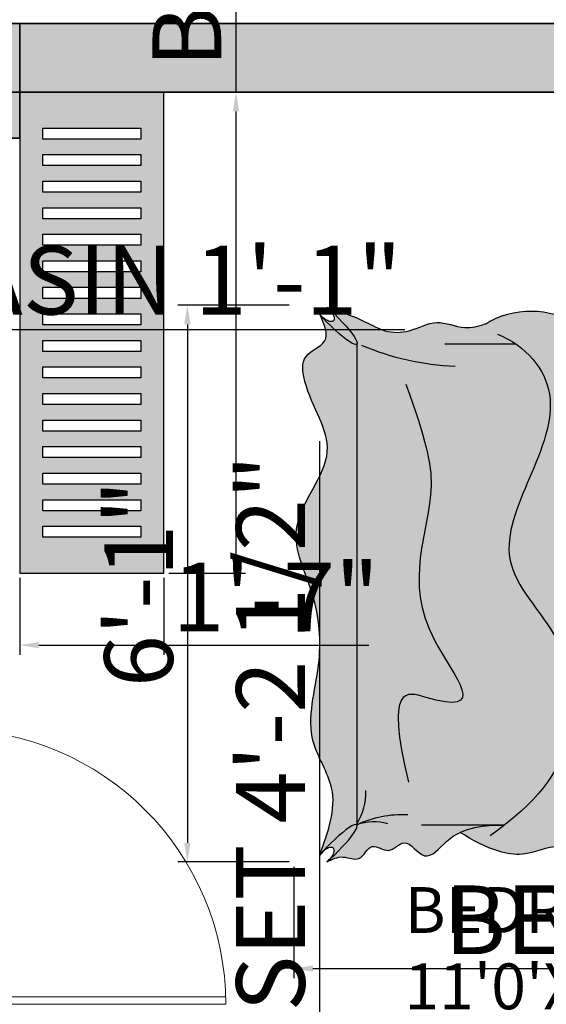
# Model space of a CAD drawing. Units: inches. Extents: x 3148 to 3962, y 1142 to 1671.
# Tile 4 of 9: x 3344 to 3413, y 1426 to 1555. Entities that reach past the tile are written whole.
import ezdxf

# ---------------------------------------------------------------- set-up
doc = ezdxf.new("R2010")
doc.units = ezdxf.units.IN
for name, color, linetype, lineweight in [('A-ANNO-DIMS', 2, 'Continuous', 18), ('A-AREA-IDEN', 7, 'Continuous', 18), ('A-COLS', 1, 'Continuous', 35), ('A-DOOR', 3, 'Continuous', 18), ('A-FURN', 8, 'Continuous', 18), ('A-WALL', 7, 'Continuous', 35), ('estofado', 7, 'Continuous', 25)]:
    doc.layers.add(name, color=color, linetype=linetype, lineweight=lineweight)
doc.layers.add('A-WALL-PATT', color=252, linetype='Continuous', lineweight=13, true_color=0x939598)
doc.layers.add('MESA', color=7, linetype='Continuous')
doc.styles.get("Standard").update_dxf_attribs({"font": 'arial.ttf'})
doc.dimstyles.new('ISO-25', dxfattribs={"dimtxt": 9, "dimasz": 2.5, "dimexe": 1.25, "dimexo": 0.625, "dimtad": 1, "dimdec": 1, "dimlunit": 3, "dimtxsty": 'Standard', "dimcen": 2.5, "dimadec": 0, "dimazin": 0, "dimtfac": 1, "dimtdec": 1, "dimtmove": 0, "dimatfit": 3, "dimfxl": 1, "dimarcsym": 0})

# ---------------------------------------------------------------- blocks, each defined once
blk = doc.blocks.new('Banco Lintz')
at = {"layer": 'MESA', "ltscale": 0.05}
h = blk.add_hatch(color=256, dxfattribs=at)
h.dxf.hatch_style = 1
h.set_gradient(color1=(138, 84, 66), color2=(0, 0, 0), one_color=1, name='INVCYLINDER')
h.paths.add_polyline_path([(0.4800000000000182, 0), (0, -5.68e-14), (0, -1.600000000000079), (0.4800000000000182, -1.600000000000079)])
h.paths.add_polyline_path([(0.403418045995295, -0.5090567265236814), (0.0765819540050643, -0.5090567265236245), (0.076581954005178, -0.4724032111287216), (0.4034180459950676, -0.4724032111288921)], flags=16)
h.paths.add_polyline_path([(0.4034180459950676, -0.5607660771784709), (0.4034180459950676, -0.597419592573317), (0.076581954005178, -0.597419592573317), (0.076581954005178, -0.560766077178414)], flags=16)
h.paths.add_polyline_path([(0.4034180459951813, -0.420693860473989), (0.0765819540050643, -0.420693860473989), (0.076581954005178, -0.3840403450791427), (0.4034180459950676, -0.3840403450791427)], flags=16)
h.paths.add_polyline_path([(0.4034180459950676, -0.6491289432280496), (0.4034180459950676, -0.6857824586229527), (0.076581954005178, -0.6857824586229527), (0.0765819540050643, -0.6491289432281065)], flags=16)
h.paths.add_polyline_path([(0.4034180459949539, -0.3323309944244102), (0.076581954005178, -0.3323309944244102), (0.0765819540050643, -0.2956774790295071), (0.4034180459950676, -0.2956774790295071)], flags=16)
h.paths.add_polyline_path([(0.4034180459950676, -0.737491809277742), (0.4034180459950676, -0.7741453246725883), (0.076581954005178, -0.7741453246725883), (0.0765819540050643, -0.737491809277742)], flags=16)
h.paths.add_polyline_path([(0.4034180459950676, -0.2439681283747745), (0.076581954005178, -0.2439681283747177), (0.076581954005178, -0.2073146129798147), (0.4034180459950676, -0.2073146129799284)], flags=16)
h.paths.add_polyline_path([(0.4034180459950676, -0.8258546753271502), (0.4034180459950676, -0.8625081907222238), (0.076581954005178, -0.86250819072211), (0.0765819540050643, -0.8258546753274913)], flags=16)
h.paths.add_polyline_path([(0.4034180459951813, -0.1556052623250821), (0.0765819540050643, -0.1556052623250252), (0.0765819540049506, -0.1189517469303496), (0.4034180459951813, -0.1189517469302928)], flags=16)
h.paths.add_polyline_path([(0.4034180459950676, -0.9142175413771269), (0.4034180459949539, -0.9508710567719163), (0.076581954005178, -0.9508710567718026), (0.076581954005178, -0.9142175413769564)], flags=16)
h.paths.add_polyline_path([(0.4034180459950676, -1.002580407426705), (0.4034180459951813, -1.039233922821438), (0.0765819540050643, -1.039233922821438), (0.076581954005178, -1.002580407426592)], flags=16)
h.paths.add_polyline_path([(0.4034180459950676, -1.090943273476284), (0.4034180459950676, -1.127596788871073), (0.076581954005178, -1.127596788871016), (0.0765819540049506, -1.090943273476284)], flags=16)
h.paths.add_polyline_path([(0.4034180459950676, -1.17930613952592), (0.4034180459950676, -1.215959654920709), (0.076581954005178, -1.215959654920709), (0.076581954005178, -1.179306139525806)], flags=16)
h.paths.add_polyline_path([(0.4034180459950676, -1.267669005575498), (0.4034180459950676, -1.304322520970401), (0.076581954005178, -1.304322520970345), (0.076581954005178, -1.267669005575498)], flags=16)
h.paths.add_polyline_path([(0.4034180459950676, -1.356031871625077), (0.4034180459950676, -1.392685387020094), (0.076581954005178, -1.39268538701998), (0.076581954005178, -1.356031871625134)], flags=16)
h.paths.add_polyline_path([(0.4034180459950676, -1.444394737673064), (0.4034180459950676, -1.481048253069729), (0.076581954005178, -1.481048253069616), (0.076581954005178, -1.444394737674826)], flags=16)
for points in [[(0, -1.600000000000022), (0.4800000000000182, -1.600000000000022), (0.4800000000000182, 0), (0, 0)], [(0.0765819540050643, -0.1189517469302928), (0.4034180459950676, -0.1189517469302928), (0.4034180459950676, -0.1556052623251389), (0.0765819540050643, -0.1556052623251389)], [(0.0765819540050643, -0.2073146129799284), (0.4034180459950676, -0.2073146129799284), (0.4034180459950676, -0.2439681283747745), (0.0765819540050643, -0.2439681283747745)], [(0.0765819540050643, -0.295677479029564), (0.4034180459950676, -0.295677479029564), (0.4034180459950676, -0.3323309944244102), (0.0765819540050643, -0.3323309944244102)], [(0.0765819540050643, -0.3840403450791996), (0.4034180459950676, -0.3840403450791996), (0.4034180459950676, -0.4206938604740458), (0.0765819540050643, -0.4206938604740458)], [(0.0765819540050643, -0.4724032111288352), (0.4034180459950676, -0.4724032111288352), (0.4034180459950676, -0.5090567265236814), (0.0765819540050643, -0.5090567265236814)], [(0.0765819540050643, -0.5607660771784709), (0.4034180459950676, -0.5607660771784709), (0.4034180459950676, -0.597419592573317), (0.0765819540050643, -0.597419592573317)], [(0.0765819540050643, -0.6491289432281065), (0.4034180459950676, -0.6491289432281065), (0.4034180459950676, -0.6857824586229527), (0.0765819540050643, -0.6857824586229527)], [(0.0765819540050643, -0.737491809277742), (0.4034180459950676, -0.737491809277742), (0.4034180459950676, -0.7741453246725883), (0.0765819540050643, -0.7741453246725883)], [(0.0765819540050643, -0.8258546753273776), (0.4034180459950676, -0.8258546753273776), (0.4034180459950676, -0.8625081907222238), (0.0765819540050643, -0.8625081907222238)], [(0.0765819540050643, -0.9142175413770132), (0.4034180459950676, -0.9142175413770132), (0.4034180459950676, -0.9508710567718593), (0.0765819540050643, -0.9508710567718593)], [(0.0765819540050643, -1.002580407426648), (0.4034180459950676, -1.002580407426648), (0.4034180459950676, -1.039233922821495), (0.0765819540050643, -1.039233922821495)], [(0.0765819540050643, -1.090943273476284), (0.4034180459950676, -1.090943273476284), (0.4034180459950676, -1.12759678887113), (0.0765819540050643, -1.12759678887113)], [(0.0765819540050643, -1.17930613952592), (0.4034180459950676, -1.17930613952592), (0.4034180459950676, -1.215959654920766), (0.0765819540050643, -1.215959654920766)], [(0.0765819540050643, -1.267669005575555), (0.4034180459950676, -1.267669005575555), (0.4034180459950676, -1.304322520970401), (0.0765819540050643, -1.304322520970401)], [(0.0765819540050643, -1.356031871625191), (0.4034180459950676, -1.356031871625191), (0.4034180459950676, -1.392685387020037), (0.0765819540050643, -1.392685387020037)], [(0.0765819540050643, -1.444394737674826), (0.4034180459950676, -1.444394737674826), (0.4034180459950676, -1.481048253069673), (0.0765819540050643, -1.481048253069673)]]:
    blk.add_lwpolyline(points, close=True, dxfattribs=at)
blk = doc.blocks.new('Cama Box Regencia LOLA')
at = {"layer": 'estofado', "ltscale": 0.2}
h = blk.add_hatch(color=256, dxfattribs=at)
h.dxf.hatch_style = 1
h.set_gradient(color1=(206, 178, 131), color2=(233, 221, 200), one_color=1, tint=0.8500000238418579, name='CURVED')
edge = h.paths.add_edge_path()
edge.add_spline(control_points=[(0.9233883396182136, -2.254908822900802), (0.9143712174658276, -2.237158585978875), (0.8971704820246486, -2.20329887728792), (0.9295105801843419, -2.140290914518345), (0.848651568119294, -2.10957861148239), (0.9047062348403186, -2.046222426005954), (0.8299480774321636, -1.990932361540615), (0.9387479200587449, -1.92692496801726), (0.8590435458045249, -1.86767849203585), (0.8322262745575699, -1.826028043643361), (0.8247981799574972, -1.810442049687992)], knot_values=[0, 0, 0, 0, 0.0575832900035364, 0.1098437972159638, 0.1698138218664432, 0.2255174829302509, 0.2824861515521905, 0.3632291183773252, 0.4509842065695901, 0.5012091817853866, 0.5012091817853866, 0.5012091817853866, 0.5012091817853866], degree=3, periodic=0)
edge.add_spline(control_points=[(0.8247981799572698, -1.810442049688447), (0.8512430237993839, -1.769990096378137), (0.8869160776755506, -1.705010622333873), (0.9070359522544322, -1.586338752195842), (0.8536462472426364, -1.488247672851343), (0.8944567470317679, -1.387739666353695), (0.8643796102055603, -1.342420998864781), (0.8547271521993025, -1.327877176513538)], knot_values=[0, 0, 0, 0, 0.1438744691785906, 0.2224893870322766, 0.3492927143212738, 0.4561786976395368, 0.5066917301592304, 0.5066917301592304, 0.5066917301592304, 0.5066917301592304], degree=3, periodic=0)
edge.add_spline(control_points=[(0.8547271521993025, -1.327877176513538), (0.7873766543807506, -1.256744909425322), (0.6449024721503065, -1.106270719748692), (0.3977250465933366, -1.412092721352792), (0.0338148848931041, -1.279726484458706), (-0.3488365122128698, -1.179158668568902), (-0.6188339616464873, -1.25080943574278), (-0.7460155200169539, -1.321708019985464)], knot_values=[0.0991852523588446, 0.0991852523588446, 0.0991852523588446, 0.0991852523588446, 0.3453008654366167, 0.6198216521345741, 0.9826525916749167, 1.386093159660275, 1.810554634340498, 1.810554634340498, 1.810554634340498, 1.810554634340498], degree=3, periodic=0)
edge.add_spline(control_points=[(-0.7460155199962628, -1.32170802000337), (-0.8056354908857201, -1.352141651537124), (-0.8226532004149476, -1.367823298399059), (-0.8348745804664758, -1.38184410903591)], knot_values=[0.0062456970656236, 0.0062456970656236, 0.0062456970656236, 0.0062456970656236, 0.0554759259147193, 0.0554759259147193, 0.0554759259147193, 0.0554759259147193], degree=3, periodic=0)
edge.add_spline(control_points=[(-0.8348745804664758, -1.38184410903591), (-0.8364250716851984, -1.383622888820184), (-0.8378983647115774, -1.385374937005849), (-0.8393716577378427, -1.387126985191514)], knot_values=[0, 0, 0, 0, 0.0062456970656236, 0.0062456970656236, 0.0062456970656236, 0.0062456970656236], degree=3, periodic=0)
edge.add_arc((-0.6180450437709624, -1.576392779500167), 0.2912164331649039, 139.4648411061637, 203.3711573294546)
edge.add_arc((-0.7011750866292914, -1.609837078845487), 0.2016528082906132, 204.0179006417974, 212.6189639884946)
edge.add_spline(control_points=[(-0.8710220093900034, -1.718537943240505), (-0.8696870122217887, -1.721658691442996), (-0.8597709916446092, -1.746046247230935), (-0.8464685798230674, -1.804421032451443), (-0.888988689927828, -1.889951451602371), (-0.8378676506146121, -1.973422824210047), (-0.8371590179440318, -2.05992368952792), (-0.8871569320951948, -2.144598622072578), (-0.908935644436724, -2.210906123939594), (-0.9233883398977695, -2.254908823284267)], knot_values=[0, 0, 0, 0, 0.0101500649009363, 0.0785829584511912, 0.1732273504791735, 0.2688802694005398, 0.3498050162211252, 0.4202002266429896, 0.5590752189863636, 0.5590752189863636, 0.5590752189863636, 0.5590752189863636], degree=3, periodic=0)
edge.add_ellipse((-0.9040800600764669, -2.258882422916315), major_axis=(0.0267880171833212, 0.0267880171833213), ratio=0.4535320972039226, start_angle=94.15910660291303, end_angle=123.37101895145429, ccw=False)
edge.add_ellipse((-0.8772920428931456, -2.232094405732993), major_axis=(0.0772920428927364, 0.0772920428927364), ratio=0.168252450050839, start_angle=-1.0527401173021644e-10, end_angle=156.3071135567154, ccw=False)
edge.add_line((-0.8000000000002955, -2.154802362840428), (0.7999592378284888, -2.154802362840428))
edge.add_arc((0.9462065466516378, -2.098298447668867), 0.1567831871334379, 200.9447658774159, 201.1244713640487, ccw=False)
edge.add_arc((1.115979327553759, -2.004946707326951), 0.3497136727815615, 205.2898146244752, 205.3730108333857)
edge.add_ellipse((0.8772920428930319, -2.232094405732993), major_axis=(-0.0772920428927364, 0.0772920428927364), ratio=0.168252450050839, start_angle=203.6928864432847, end_angle=359.99999999994674, ccw=False)
edge.add_ellipse((0.9040800600763532, -2.258882422916315), major_axis=(-0.0267880171833213, 0.0267880171833213), ratio=0.4535320972039226, start_angle=236.6289810485458, end_angle=265.84089339708703, ccw=False)
h = blk.add_hatch(color=256, dxfattribs=at)
h.dxf.hatch_style = 1
h.set_gradient(color1=(206, 178, 131), color2=(233, 221, 200), one_color=1, tint=0.8500000238418579, name='CURVED')
edge = h.paths.add_edge_path()
edge.add_ellipse((-0.8772920428931456, -2.232094405732993), major_axis=(0.0772920428927364, 0.0772920428927364), ratio=0.168252450050839, start_angle=-156.3071135577263, end_angle=-1.05349e-10)
edge.add_ellipse((-0.8772920428931456, -2.232094405732993), major_axis=(0.0772920428927364, 0.0772920428927364), ratio=0.168252450050839, start_angle=-1.05349e-10, end_angle=156.3071135567153)
edge.add_ellipse((-0.9040800600764669, -2.258882422916315), major_axis=(0.0267880171833212, 0.0267880171833213), ratio=0.4535320972039226, start_angle=-94.15910660848522, end_angle=94.15910660291303, ccw=False)
h = blk.add_hatch(color=256, dxfattribs=at)
h.dxf.hatch_style = 1
h.set_gradient(color1=(206, 178, 131), color2=(233, 221, 200), one_color=1, tint=0.8500000238418579, name='CURVED')
edge = h.paths.add_edge_path()
edge.add_spline(control_points=[(-0.9001064604443627, -2.27819070273756), (-0.866259371332262, -2.263084355976445), (-0.8028331991894219, -2.234776522858453), (-0.7685206103102474, -2.343981002846874), (-0.6122536186376238, -2.322828464485212), (-0.4353754265674752, -2.183795504726106), (-0.2043351766035357, -2.412166101990749), (0.035742157155596, -2.28434544697319), (0.2724023732024534, -2.265741378418681), (0.4990197572961961, -2.339647395113615), (0.6925408411253784, -2.202138696866825), (0.8240737498149427, -2.250332331133733), (0.900106460444249, -2.27819070273756)], knot_values=[0, 0, 0, 0, 0.0915194039844232, 0.1714985135733706, 0.2551966802733756, 0.4993431682155844, 0.7776132872898075, 0.9991109890269537, 1.23769004728933, 1.492615491211055, 1.658192352121012, 1.885025012049534, 1.885025012049534, 1.885025012049534, 1.885025012049534], degree=3, periodic=0)
edge.add_ellipse((0.9040800600763532, -2.258882422916315), major_axis=(-0.0267880171833213, 0.0267880171833213), ratio=0.4535320972039226, start_angle=454.1591066084853, end_angle=483.3710189511271, ccw=False)
edge.add_ellipse((0.8772920428930319, -2.232094405732993), major_axis=(-0.0772920428927364, 0.0772920428927364), ratio=0.168252450050839, start_angle=359.99999999994674, end_angle=516.3071135577263, ccw=False)
edge.add_arc((0.9462065466977946, -2.098298447788181), 0.1567831871334379, 201.1244713173118, 201.142614633458, ccw=False)
edge.add_line((0.7999592378286025, -2.154802362840428), (-0.8000000000004092, -2.154802362840428))
edge.add_ellipse((-0.8772920428931456, -2.232094405732993), major_axis=(0.0772920428927364, 0.0772920428927364), ratio=0.168252450050839, start_angle=-156.3071135577261, end_angle=-1.0527401173021644e-10, ccw=False)
edge.add_ellipse((-0.9040800600764669, -2.258882422916315), major_axis=(0.0267880171833212, 0.0267880171833213), ratio=0.4535320972039226, start_angle=-123.3710189511271, end_angle=-94.15910660848522, ccw=False)
h = blk.add_hatch(color=256, dxfattribs=at)
h.dxf.hatch_style = 1
h.set_gradient(color1=(206, 178, 131), color2=(233, 221, 200), one_color=1, tint=0.8500000238418579, name='CURVED')
edge = h.paths.add_edge_path()
edge.add_ellipse((0.8772920428930319, -2.232094405732993), major_axis=(-0.0772920428927364, 0.0772920428927364), ratio=0.168252450050839, start_angle=203.6928864432846, end_angle=359.9999999999468)
edge.add_ellipse((0.8772920428930319, -2.232094405732993), major_axis=(-0.0772920428927364, 0.0772920428927364), ratio=0.168252450050839, start_angle=359.9999999999468, end_angle=516.3071135577261)
edge.add_ellipse((0.9040800600763532, -2.258882422916315), major_axis=(-0.0267880171833213, 0.0267880171833213), ratio=0.4535320972039226, start_angle=265.84089339708703, end_angle=454.1591066084853, ccw=False)
for p, q in [((-0.7999999999999546, -1.624303127646271), (-0.7999999999999546, -1.862122701256737)), ((0.8000000000000682, -1.939064283336335), (0.8000000000000682, -1.662039728679133)), ((-0.7999999999999546, -2.154802362840428), (0.8000000000000682, -2.154802362840428))]:
    blk.add_line(p, q, dxfattribs=at)
for centre, radius, start, end in [((-0.618045043771076, -1.576392779500224), 0.2912164331649248, 139.4648411061415, 203.3711573294531), ((-0.7011750866354305, -1.609837078830935), 0.2016528082909061, 204.017900646285, 212.6189640158667), ((-1.599544017339439, -1.795539319485669), 0.8732121282601557, 336.8495239496693, 357.9002538876362), ((1.115979327644367, -2.00494670751874), 0.3497136727815545, 176.7524727679717, 205.3730107986517), ((0.9462065466502735, -2.098298447665399), 0.1567831871334492, 162.6474673821321, 201.1361021892849), ((0.6916068347399005, -2.322769188842187), 0.1980600766927276, 58.0012856468178, 91.6550645032879)]:
    blk.add_arc(centre, radius, start, end, dxfattribs=at)
at = {"layer": 'estofado', "ltscale": 0.2, "extrusion": (0, 0, -1)}
for centre, major_axis, ratio, start_param, end_param in [((-0.8772920428931456, -2.232094405732993), (0.0772920428927364, 0.0772920428927364), 0.168252450050839, 4.250341947992563, 8.31602866635556), ((-0.9040800600764669, -2.258882422916315), (0.0267880171833212, 0.0267880171833213), 0.4535320972039226, 4.422106649467695, 8.144263964888069)]:
    blk.add_ellipse(centre, major_axis=major_axis, ratio=ratio, start_param=start_param, end_param=end_param, dxfattribs=at)
at = {"layer": 'estofado', "ltscale": 0.2}
for centre, major_axis, ratio, start_param, end_param in [((0.8772920428930319, -2.232094405732993), (-0.0772920428927364, 0.0772920428927364), 0.168252450050839, 4.250341947992563, 8.31602866635556), ((0.9040800600763532, -2.258882422916315), (-0.0267880171833213, 0.0267880171833213), 0.4535320972039226, 4.422106649467695, 8.144263964888069)]:
    blk.add_ellipse(centre, major_axis=major_axis, ratio=ratio, start_param=start_param, end_param=end_param, dxfattribs=at)
for points, knots in [([(0.8547271521993025, -1.327877176513538), (0.8643796102055603, -1.342420998864781), (0.8944567470317679, -1.387739666353695), (0.8536462472426364, -1.488247672851343), (0.9070359522544322, -1.586338752195842), (0.8869160776755506, -1.705010622333873), (0.8512430237993839, -1.769990096378137), (0.8247981799572698, -1.810442049688447)], [0, 0, 0, 0, 0.0505130325196935, 0.1573990158379565, 0.2842023431269537, 0.3628172609806397, 0.5066917301592304, 0.5066917301592304, 0.5066917301592304, 0.5066917301592304]), ([(-0.8337777191962914, -1.686127396833001), (-0.7936227331957753, -1.590003258421234), (-0.5563859991466416, -1.394748990587913), (-0.1321102153461879, -1.783182047565389), (0.1908245506583626, -1.429131816234075), (0.5373208507353411, -1.424480211867205), (0.720102724937533, -1.549855593291283), (0.836774155394778, -1.71068108627179)], [0.0299011711635954, 0.0299011711635954, 0.0299011711635954, 0.0299011711635954, 0.2769669118207226, 0.7971145189980146, 1.093669199334649, 1.464665995707328, 1.788488893467898, 1.788488893467898, 1.788488893467898, 1.788488893467898]), ([(0.9233883396182136, -2.254908822900802), (0.9143712174658222, -2.237158585978864), (0.8971704820247243, -2.203298877287874), (0.9295105801841641, -2.140290914518474), (0.8486515681193482, -2.109578611482328), (0.9047062348404182, -2.046222426005942), (0.8299480774320162, -1.990932361540672), (0.9387479200587655, -1.926924968017257), (0.8039686482702052, -1.826739790434252), (0.8016292922223446, -1.72965583153342), (0.8000000000000682, -1.662039728679133)], [0, 0, 0, 0, 0.0575832900035364, 0.1098437972159638, 0.1698138218664432, 0.2255174829302509, 0.2824861515521905, 0.3632291183773252, 0.4509842065695901, 0.6523445315224259, 0.6523445315224259, 0.6523445315224259, 0.6523445315224259]), ([(-0.9233883398977695, -2.254908823284267), (-0.908935644436724, -2.210906123939594), (-0.8871569320951948, -2.144598622072578), (-0.8371590179440318, -2.05992368952792), (-0.8378676506146121, -1.973422824210047), (-0.888988689927828, -1.889951451602371), (-0.8464685798230674, -1.804421032451443), (-0.8597709916446092, -1.746046247230935), (-0.8696870122217887, -1.721658691442996), (-0.8710220093900034, -1.718537943240505)], [0, 0, 0, 0, 0.1388749923433741, 0.2092702027652384, 0.2901949495858238, 0.3858478685071901, 0.4804922605351724, 0.5489251540854273, 0.5590752189863636, 0.5590752189863636, 0.5590752189863636, 0.5590752189863636]), ([(-0.6667836004502306, -1.991594303623287), (-0.4801926263546648, -1.924290517138388), (-0.2421721137753821, -1.866692280098163), (0.067250899423243, -2.056782250863193), (0.4752270537671848, -1.673138005031375), (0.3282580065483671, -2.063228784622481), (0.6572625331713198, -1.982435509858419)], [0.0299011711635954, 0.0299011711635954, 0.0299011711635954, 0.0299011711635954, 0.2769669118207226, 0.7971145189980146, 1.093669199334649, 1.16835959978728, 1.16835959978728, 1.16835959978728, 1.16835959978728]), ([(0.900106460444249, -2.27819070273756), (0.8240737498147286, -2.250332331133789), (0.6925408411252015, -2.202138696866918), (0.4990197572963532, -2.33964739511349), (0.2724023732023884, -2.265741378418779), (0.0357421571555867, -2.284345446973105), (-0.204335176603578, -2.412166101990773), (-0.4353754265674596, -2.183795504726199), (-0.6122536186375224, -2.322828464485116), (-0.7685206103102122, -2.343981002846907), (-0.8028331991894692, -2.234776522858419), (-0.8662593713322198, -2.263084355976456), (-0.9001064604443627, -2.27819070273756)], [0, 0, 0, 0, 0.2268326599285221, 0.3924095208384793, 0.6473349647602045, 0.8859140230225809, 1.107411724759727, 1.38568184383395, 1.629828331776159, 1.713526498476164, 1.793505608065111, 1.885025012049534, 1.885025012049534, 1.885025012049534, 1.885025012049534])]:
    blk.add_open_spline(points, degree=3, knots=knots, dxfattribs=at)
blk = doc.blocks.new('*D42')
at = {"layer": 'A-ANNO-DIMS', "color": 0, "lineweight": -2, "transparency": 16777216}
for p, q in [((3194.042306275787, 1555.424200034517), (3194.042306275787, 1571.690472151851)), ((3482.042306275788, 1555.424200034517), (3482.042306275788, 1571.690472151851)), ((3196.542306275788, 1570.440472151851), (3479.542306275788, 1570.440472151851))]:
    blk.add_line(p, q, dxfattribs=at)
at = {"layer": 'A-ANNO-DIMS', "color": 0, "transparency": 16777216}
for points in [[(3196.542306275788, 1570.857138818518), (3196.542306275788, 1570.023805485184), (3194.042306275787, 1570.440472151851)], [(3479.542306275788, 1570.857138818518), (3479.542306275788, 1570.023805485184), (3482.042306275788, 1570.440472151851)]]:
    blk.add_solid(points, dxfattribs=at)
at = {"layer": 'Defpoints', "color": 0, "transparency": 16777216}
for p in [(3482.042306275788, 1570.440472151851), (3194.042306275787, 1554.799200034517), (3482.042306275788, 1554.799200034517)]:
    blk.add_point(p, dxfattribs=at)
at = {"layer": 'A-ANNO-DIMS', "color": 0, "transparency": 16777216, "insert": (3338.042306275787, 1575.583889614334), "char_height": 9, "attachment_point": 5}
blk.add_mtext("24'", dxfattribs=at)
blk = doc.blocks.new('DOOR-SWING-36')
for p, q in [((35.98610843089318, 1.000000000000227), (0, 1.000000000000227)), ((0, 2.274e-13), (0, 1.000000000000227)), ((36, 2.274e-13), (0, 2.274e-13))]:
    blk.add_line(p, q)
blk.add_arc((0, 2.274e-13), 36, 0, 90)
blk = doc.blocks.new('COL-9X15')
h = blk.add_hatch(color=256)
h.dxf.hatch_style = 1
h.paths.add_polyline_path([(9.000306275787352, 15.00020003451709), (0.0003062757873522, 15.00020003451709), (0.0003062757873522, 0.0002000345170927), (9.000306275787352, 0.0002000345170927)])
blk.add_lwpolyline([(9.000306275787352, 0.0002000345170927), (9.000306275787352, 15.00020003451709), (0.0003062757873522, 15.00020003451709), (0.0003062757873522, 0.0002000345170927)], close=True)
blk = doc.blocks.new('*D92')
at = {"layer": 'A-ANNO-DIMS', "color": 0, "lineweight": -2, "transparency": 16777216}
for p, q in [((3372.388778275791, 1545.799200034518), (3372.388778275791, 1620.579213677083)), ((3363.564954275789, 1545.799200034518), (3373.638778275792, 1545.799200034518)), ((3372.388778275791, 1485.307040034514), (3372.388778275791, 1543.299200034518)), ((3363.564954275789, 1482.807040034514), (3373.638778275792, 1482.807040034514))]:
    blk.add_line(p, q, dxfattribs=at)
at = {"layer": 'A-ANNO-DIMS', "color": 0, "transparency": 16777216}
for points in [[(3371.972111609125, 1543.299200034518), (3372.805444942458, 1543.299200034518), (3372.388778275791, 1545.799200034518)], [(3371.972111609125, 1485.307040034514), (3372.805444942458, 1485.307040034514), (3372.388778275791, 1482.807040034514)]]:
    blk.add_solid(points, dxfattribs=at)
at = {"layer": 'Defpoints', "color": 0, "transparency": 16777216}
for p in [(3362.93995427579, 1545.799200034518), (3372.388778275791, 1545.799200034518), (3362.93995427579, 1482.807040034514)]:
    blk.add_point(p, dxfattribs=at)
at = {"layer": 'A-ANNO-DIMS', "color": 0, "transparency": 16777216, "insert": (3367.107229844686, 1584.439206855799), "char_height": 9, "attachment_point": 5, "rotation": 90}
blk.add_mtext('BENCH 5\'-3"', dxfattribs=at)
blk = doc.blocks.new('*D93')
at = {"layer": 'A-ANNO-DIMS', "color": 0, "lineweight": -2, "transparency": 16777216}
for p, q in [((3344.042306275787, 1482.182040034514), (3344.042306275787, 1472.108216034513)), ((3362.939954275788, 1482.182040034514), (3362.939954275788, 1472.108216034513)), ((3346.542306275787, 1473.358216034513), (3360.439954275788, 1473.358216034513)), ((3362.939954275788, 1473.358216034513), (3389.76703476692, 1473.358216034513))]:
    blk.add_line(p, q, dxfattribs=at)
at = {"layer": 'A-ANNO-DIMS', "color": 0, "transparency": 16777216}
for points in [[(3346.542306275787, 1473.77488270118), (3346.542306275787, 1472.941549367847), (3344.042306275787, 1473.358216034513)], [(3360.439954275788, 1473.77488270118), (3360.439954275788, 1472.941549367847), (3362.939954275788, 1473.358216034513)]]:
    blk.add_solid(points, dxfattribs=at)
at = {"layer": 'Defpoints', "color": 0, "transparency": 16777216}
for p in [(3344.042306275787, 1482.807040034514), (3362.939954275788, 1482.807040034514), (3362.939954275788, 1473.358216034513)]:
    blk.add_point(p, dxfattribs=at)
at = {"layer": 'A-ANNO-DIMS', "color": 0, "transparency": 16777216, "insert": (3377.603494521354, 1478.501633496996), "char_height": 9, "attachment_point": 5}
blk.add_mtext('1\'-7"', dxfattribs=at)
blk = doc.blocks.new('*D94')
at = {"layer": 'A-ANNO-DIMS', "color": 0, "lineweight": -2, "transparency": 16777216}
for p, q in [((3379.971676630814, 1444.320308753911), (3379.971676630814, 1429.734714307165)), ((3473.042306275787, 1444.320308753911), (3473.042306275787, 1429.734714307165)), ((3382.471676630814, 1430.984714307166), (3470.542306275787, 1430.984714307166))]:
    blk.add_line(p, q, dxfattribs=at)
at = {"layer": 'A-ANNO-DIMS', "color": 0, "transparency": 16777216}
for points in [[(3382.471676630814, 1431.401380973832), (3382.471676630814, 1430.568047640499), (3379.971676630814, 1430.984714307166)], [(3470.542306275787, 1431.401380973832), (3470.542306275787, 1430.568047640499), (3473.042306275787, 1430.984714307166)]]:
    blk.add_solid(points, dxfattribs=at)
at = {"layer": 'Defpoints', "color": 0, "transparency": 16777216}
for p in [(3379.971676630814, 1444.945308753911), (3473.042306275787, 1444.945308753911), (3473.042306275787, 1430.984714307166)]:
    blk.add_point(p, dxfattribs=at)
at = {"layer": 'A-ANNO-DIMS', "color": 0, "transparency": 16777216, "insert": (3426.506991453301, 1436.204871196661), "char_height": 9, "attachment_point": 5}
blk.add_mtext('BED 7\'-9"', dxfattribs=at)
blk = doc.blocks.new('*D95')
at = {"layer": 'A-ANNO-DIMS', "color": 0, "lineweight": -2, "transparency": 16777216}
for p, q in [((3379.346676630816, 1517.89242109905), (3364.761082184071, 1517.89242109905)), ((3366.011082184071, 1515.39242109905), (3366.011082184071, 1447.445308753912)), ((3379.346676630816, 1444.945308753912), (3364.761082184071, 1444.945308753912))]:
    blk.add_line(p, q, dxfattribs=at)
at = {"layer": 'A-ANNO-DIMS', "color": 0, "transparency": 16777216}
for points in [[(3365.594415517404, 1515.39242109905), (3366.427748850738, 1515.39242109905), (3366.011082184071, 1517.89242109905)], [(3365.594415517404, 1447.445308753912), (3366.427748850738, 1447.445308753912), (3366.011082184071, 1444.945308753912)]]:
    blk.add_solid(points, dxfattribs=at)
at = {"layer": 'Defpoints', "color": 0, "transparency": 16777216}
for p in [(3379.971676630816, 1517.89242109905), (3366.011082184071, 1444.945308753912), (3379.971676630816, 1444.945308753912)]:
    blk.add_point(p, dxfattribs=at)
at = {"layer": 'A-ANNO-DIMS', "color": 0, "transparency": 16777216, "insert": (3360.790925294575, 1481.41886492648), "char_height": 9, "attachment_point": 5, "rotation": 90}
blk.add_mtext('6\'-1"', dxfattribs=at)
blk = doc.blocks.new('*D96')
at = {"layer": 'A-ANNO-DIMS', "color": 0, "lineweight": -2, "transparency": 16777216}
for p, q in [((3383.348513637209, 1376.460949868962), (3383.348513637209, 1500.102491478784)), ((3390.322161525081, 1376.460949868962), (3382.09851363721, 1376.460949868962)), ((3383.348513637209, 1328.303297283138), (3383.348513637209, 1373.960949868962)), ((3390.322161525081, 1325.803297283138), (3382.09851363721, 1325.803297283138))]:
    blk.add_line(p, q, dxfattribs=at)
at = {"layer": 'A-ANNO-DIMS', "color": 0, "transparency": 16777216}
for points in [[(3382.931846970543, 1373.960949868962), (3383.765180303876, 1373.960949868962), (3383.348513637209, 1376.460949868962)], [(3382.931846970543, 1328.303297283138), (3383.765180303876, 1328.303297283138), (3383.348513637209, 1325.803297283138)]]:
    blk.add_solid(points, dxfattribs=at)
at = {"layer": 'Defpoints', "color": 0, "transparency": 16777216}
for p in [(3383.348513637209, 1376.460949868962), (3390.947161525081, 1376.460949868962), (3390.947161525081, 1325.803297283138)]:
    blk.add_point(p, dxfattribs=at)
at = {"layer": 'A-ANNO-DIMS', "color": 0, "transparency": 16777216, "insert": (3378.070034783185, 1439.531720673872), "char_height": 9, "attachment_point": 5, "rotation": 90}
blk.add_mtext('DINING SET 4\'-2 1/2"', dxfattribs=at)
blk = doc.blocks.new('*D110')
at = {"layer": 'A-ANNO-DIMS', "color": 0, "lineweight": -2, "transparency": 16777216}
for p, q in [((3313.101746403582, 1513.424200034517), (3313.101746403582, 1515.985919170834)), ((3326.013207312363, 1513.424200034517), (3326.013207312363, 1515.985919170834)), ((3315.601746403582, 1514.735919170834), (3323.513207312363, 1514.735919170834)), ((3326.013207312363, 1514.735919170834), (3394.512866248243, 1514.735919170834))]:
    blk.add_line(p, q, dxfattribs=at)
at = {"layer": 'A-ANNO-DIMS', "color": 0, "transparency": 16777216}
for points in [[(3315.601746403582, 1515.152585837501), (3315.601746403582, 1514.319252504167), (3313.101746403582, 1514.735919170834)], [(3323.513207312363, 1515.152585837501), (3323.513207312363, 1514.319252504167), (3326.013207312363, 1514.735919170834)]]:
    blk.add_solid(points, dxfattribs=at)
at = {"layer": 'Defpoints', "color": 0, "transparency": 16777216}
for p in [(3326.013207312363, 1514.735919170834), (3313.101746403582, 1512.799200034517), (3326.013207312363, 1512.799200034517)]:
    blk.add_point(p, dxfattribs=at)
at = {"layer": 'A-ANNO-DIMS', "color": 0, "transparency": 16777216, "insert": (3361.513036780303, 1520.014398024859), "char_height": 9, "attachment_point": 5}
blk.add_mtext('BASIN 1\'-1"', dxfattribs=at)

msp = doc.modelspace()

# ---------------------------------------------------------------- hatches: boundary and pattern name
at = {"layer": 'A-WALL-PATT'}
h = msp.add_hatch(color=256, dxfattribs=at)
h.dxf.hatch_style = 1
h.paths.add_polyline_path([(3203.042306275788, 1410.799200034518), (3194.042306275787, 1410.799200034518), (3194.042306275787, 1296.799200034517), (3203.042306275786, 1296.799200034517), (3203.042306275787, 1300.855382799943)])
h.paths.add_polyline_path([(3203.042306275778, 1281.799200034517), (3194.042306275787, 1281.799200034517), (3194.042306275787, 1212.799200034517), (3203.042306275788, 1212.799200034517)])
h.paths.add_polyline_path([(3326.042306275788, 1206.799200034517), (3203.042306275788, 1206.799200034517), (3203.042306275788, 1197.799200034517), (3326.042306275788, 1197.799200034517)])
h.paths.add_polyline_path([(3341.042306275787, 1362.799200034517), (3335.042306275788, 1362.799200034517), (3335.042306275788, 1290.799200034517), (3341.042306275787, 1290.799200034517)])
h.paths.add_polyline_path([(3341.042306275788, 1207.799200034517), (3335.042306275788, 1207.799200034517), (3335.042306275788, 1206.799200034517), (3341.042306275788, 1206.799200034517)])
h.paths.add_polyline_path([(3341.042306275787, 1259.799200034517), (3335.042306275788, 1259.799200034517), (3335.042306275788, 1255.799200034517), (3341.042306275787, 1255.799200034517)])
h.paths.add_polyline_path([(3341.042306275787, 1281.799200034517), (3335.042306275788, 1281.799200034517), (3335.042306275788, 1277.799200034517), (3341.042306275787, 1277.799200034517)])
h.paths.add_polyline_path([(3377.042306275787, 1287.799200034517), (3350.042306275788, 1287.799200034517), (3350.042306275788, 1281.799200034517), (3377.042306275787, 1281.799200034517)])
h.paths.add_polyline_path([(3473.042306275787, 1287.799200034517), (3445.042307275787, 1287.799200034517), (3437.042306275787, 1287.799200034517), (3437.042306275788, 1281.799200034517), (3473.042306275787, 1281.799200034517)])
h.paths.add_polyline_path([(3482.042306275788, 1313.299200034517), (3473.042306275787, 1313.299200034517), (3473.042306275787, 1296.799200034517), (3482.042306275788, 1296.799200034517)])
h.paths.add_polyline_path([(3482.042306275788, 1410.799200034517), (3473.042306275787, 1410.799200034517), (3473.042306275787, 1385.299200034517), (3482.042306275788, 1385.299200034517)])
h.paths.add_polyline_path([(3473.042306275787, 1416.799200034517), (3344.042306275788, 1416.799200034517), (3344.042306275788, 1410.799200034517), (3473.042306275787, 1410.799200034517)])
h.paths.add_polyline_path([(3482.042306275788, 1445.299200034517), (3473.042306275787, 1445.299200034517), (3473.042306275787, 1425.799200034517), (3482.042306275788, 1425.799200034517)])
h.paths.add_polyline_path([(3341.042306275787, 1426.299200034517), (3335.042306275788, 1426.299200034517), (3335.042306275788, 1425.799200034517), (3341.042306275787, 1425.799200034517)])
h.paths.add_polyline_path([(3304.042306275788, 1428.799200034517), (3253.542306275787, 1428.799200034517), (3253.542306275788, 1430.299200034517), (3251.042306275788, 1430.299200034517), (3251.042306275787, 1428.799200034517), (3203.042306275788, 1428.799200034517), (3203.042306275788, 1512.799200034517), (3215.042306275788, 1512.799200034517), (3215.042306275788, 1518.799200034517), (3203.042306275788, 1518.799200034517), (3203.042306275788, 1539.799200034517), (3194.042306275787, 1539.799200034517), (3194.042306275787, 1425.799200034519), (3203.042306275787, 1425.799200034519), (3203.042306275787, 1422.799200034517), (3304.042306275788, 1422.799200034517)])
h.paths.add_polyline_path([(3265.542306275789, 1518.799200034517), (3239.042306275788, 1518.799200034517), (3239.042306275788, 1512.799200034517), (3251.042306275788, 1512.799200034517), (3251.042306275788, 1461.299200034517), (3253.542306275789, 1461.299200034517), (3253.542306275789, 1462.299200034517), (3255.542306275788, 1462.299200034517), (3255.542306275788, 1464.799200034517), (3253.542306275789, 1464.799200034517), (3253.542306275788, 1512.799200034517), (3265.542306275789, 1512.799200034517)], flags=17)
h.paths.add_polyline_path([(3307.542306275788, 1518.799200034517), (3289.542306275789, 1518.799200034517), (3289.542306275789, 1512.799200034517), (3301.542306275788, 1512.799200034517), (3301.542306275788, 1464.799200034517), (3286.542306275788, 1464.799200034517), (3286.542306275788, 1462.299200034517), (3304.042306275788, 1462.299200034517), (3304.042306275788, 1512.799200034517), (3307.542306275788, 1512.799200034517)])
h.paths.add_polyline_path([(3341.042306275787, 1539.799200034517), (3335.042306275788, 1539.799200034517), (3335.042306275788, 1518.799200034517), (3331.542306275788, 1518.799200034517), (3331.542306275788, 1512.799200034517), (3335.042306275788, 1512.799200034517), (3335.042306275788, 1462.299200034517), (3341.042306275787, 1462.299200034517)])
h.paths.add_polyline_path([(3335.042306275788, 1554.799200034517), (3203.042306275788, 1554.799200034517), (3203.042306275788, 1545.799200034517), (3335.042306275788, 1545.799200034517)])
h.paths.add_polyline_path([(3473.042306275787, 1554.799200034517), (3344.042306275787, 1554.799200034517), (3344.042306275787, 1545.799200034517), (3362.939954275788, 1545.799200034517), (3473.042306275787, 1545.799200034517)])
h.paths.add_polyline_path([(3482.042306275788, 1539.799200034517), (3473.042306275787, 1539.799200034517), (3473.042306275787, 1517.299200034517), (3482.042306275788, 1517.299200034517)])

# ---------------------------------------------------------------- linework, layer by layer
at = {"layer": 'A-WALL'}
for p, q in [((3194.042306275787, 1554.799200034517), (3482.042306275788, 1554.799200034517)), ((3341.042306275787, 1545.799200034517), (3473.042306275787, 1545.799200034517))]:
    msp.add_line(p, q, dxfattribs=at)

# ---------------------------------------------------------------- block references
at = {"layer": 'A-COLS'}
msp.add_blockref('COL-9X15', (3335.041999999999, 1539.799000000001), dxfattribs=at)
at = {"layer": 'A-DOOR'}
msp.add_blockref('DOOR-SWING-36', (3335.042306275787, 1426.299200034517), dxfattribs=at)
at = {"layer": 'A-FURN', "xscale": 39.3701, "yscale": 39.3701, "zscale": 39.3701}
msp.add_blockref('Banco Lintz', (3344.042306275787, 1545.799200034517), dxfattribs=at)
at = {"layer": 'A-FURN', "xscale": 39.3701, "yscale": 39.3701, "zscale": 39.3701, "rotation": 270}
msp.add_blockref('Cama Box Regencia LOLA', (3473.042306275787, 1481.299200034517), dxfattribs=at)

# ---------------------------------------------------------------- texts
at = {"layer": 'A-AREA-IDEN', "insert": (3394.465913550088, 1441.652798430895), "char_height": 6, "attachment_point": 1}
msp.add_mtext_dynamic_manual_height_columns('BEDROOM\\P11\'0\'X10\'9"', width=77.95175509674118, gutter_width=12.5, heights=[0], dxfattribs=at)

# ---------------------------------------------------------------- dimensions: what is measured, and where the dimension line sits
at = {"layer": 'A-ANNO-DIMS'}
for base, p1, p2, text, picture, middle in [((3372.388778275791, 1545.799200034518), (3362.939954275788, 1482.807040034514), (3362.939954275788, 1545.799200034517), 'BENCH <>', '*D92', (3367.107229844686, 1584.439206855799)), ((3383.348513637209, 1376.460949868962), (3390.94716152508, 1325.803297283137), (3390.94716152508, 1376.460949868961), 'DINING SET <>', '*D96', (3378.070034783185, 1439.531720673872))]:
    dim = msp.add_linear_dim(base=base, p1=p1, p2=p2, angle=90, text=text, dimstyle='ISO-25', override={"dimdec": 1, "dimlfac": 1, "dimrnd": 0, "dimzin": 1, "dimdsep": 46, "dimlunit": 4, "dimfrac": 2}, dxfattribs=at)
    dim.commit()
    dim.dimension.update_dxf_attribs({"geometry": picture, "text_midpoint": middle})
for base, p1, p2, override, picture, middle in [((3482.042306275788, 1570.440472151851), (3194.042306275787, 1554.799200034517), (3482.042306275788, 1554.799200034517), {"dimclrd": 0, "dimclre": 0, "dimclrt": 0}, '*D42', (3338.042306275787, 1575.583889614334)), ((3362.939954275788, 1473.358216034513), (3344.042306275787, 1482.807040034514), (3362.939954275788, 1482.807040034514), {"dimdec": 1, "dimlfac": 1, "dimrnd": 0, "dimzin": 1, "dimdsep": 46, "dimlunit": 4, "dimfrac": 2}, '*D93', (3377.603494521354, 1478.501633496996))]:
    dim = msp.add_linear_dim(base=base, p1=p1, p2=p2, dimstyle='ISO-25', override=override, dxfattribs=at)
    dim.commit()
    dim.dimension.update_dxf_attribs({"geometry": picture, "text_midpoint": middle})
for base, p1, p2, text, picture, middle in [((3326.013207312363, 1514.735919170834), (3313.101746403582, 1512.799200034517), (3326.013207312363, 1512.799200034517), 'BASIN <>', '*D110', (3361.513036780303, 1520.014398024859)), ((3473.042306275787, 1430.984714307166), (3379.971676630814, 1444.945308753911), (3473.042306275787, 1444.945308753911), 'BED <>', '*D94', (3426.506991453301, 1436.204871196661))]:
    dim = msp.add_linear_dim(base=base, p1=p1, p2=p2, text=text, dimstyle='ISO-25', override={"dimdec": 1, "dimlfac": 1, "dimrnd": 0, "dimzin": 1, "dimdsep": 46, "dimlunit": 4, "dimfrac": 2}, dxfattribs=at)
    dim.commit()
    dim.dimension.update_dxf_attribs({"geometry": picture, "text_midpoint": middle})
dim = msp.add_linear_dim(base=(3366.011082184071, 1444.945308753912), p1=(3379.971676630814, 1517.892421099049), p2=(3379.971676630814, 1444.945308753911), angle=270, dimstyle='ISO-25', override={"dimdec": 1, "dimlfac": 1, "dimrnd": 0, "dimzin": 1, "dimdsep": 46, "dimlunit": 4, "dimfrac": 2}, dxfattribs=at)
dim.commit()
dim.dimension.update_dxf_attribs({"geometry": '*D95', "text_midpoint": (3360.790925294575, 1481.41886492648)})

doc.saveas('drawing.dxf')
